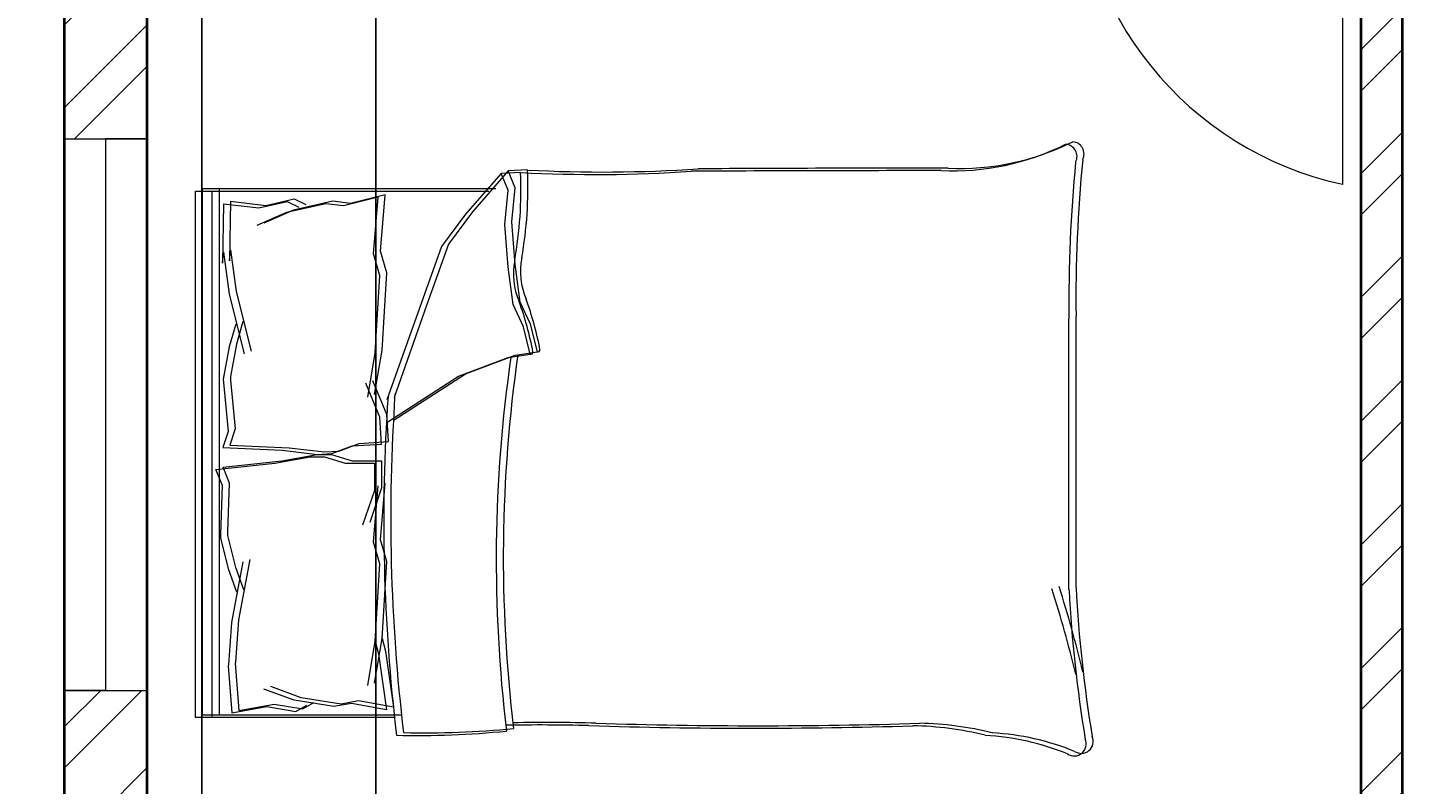
# Model space of a CAD drawing. Units: inches. Extents: x 1355 to 2746, y 1171 to 2751.
# Tile 7 of 24: x 1511 to 1663, y 1818 to 1901. Entities that reach past the tile are written whole.
import ezdxf

# ---------------------------------------------------------------- set-up
doc = ezdxf.new("R2010")
doc.units = ezdxf.units.IN
for name, color, linetype, lineweight in [('A-ANNO-DIMS', 2, 'Continuous', 18), ('A-DOOR', 3, 'Continuous', 20), ('A-FURN', 8, 'Continuous', 13), ('A-GLAZ', 4, 'Continuous', 18), ('A-WALL', 7, 'Continuous', 40), ('A-WALL-PATT', 252, 'Continuous', 13)]:
    doc.layers.add(name, color=color, linetype=linetype, lineweight=lineweight)
doc.styles.get("Standard").update_dxf_attribs({"font": 'arial.ttf'})
doc.dimstyles.get("Standard").update_dxf_attribs({"dimtxt": 0.18, "dimasz": 0.18, "dimexe": 0.18, "dimexo": 0.0625, "dimgap": 0.09, "dimtad": 0, "dimtih": 1, "dimtoh": 1, "dimdec": 4, "dimzin": 0, "dimdsep": 46, "dimtxsty": 'Standard', "dimcen": 0.09, "dimadec": 0, "dimazin": 0, "dimtfac": 1, "dimtdec": 4, "dimtofl": 0, "dimtmove": 0, "dimatfit": 3, "dimfxl": 1, "dimtolj": 1, "dimtzin": 0, "dimarcsym": 0})

# ---------------------------------------------------------------- blocks, each defined once
blk = doc.blocks.new('BED-DOUBLE-PLAN')
for p, q in [((75.16, 62.38), (96.87, 62.38)), ((75.93, 62.66), (97.64, 62.66)), ((95.03, 62.38), (95.03, 5.09)), ((95.8, 62.66), (95.8, 5.36)), ((96.87, 62.38), (96.87, 5.09)), ((97.64, 62.66), (97.64, 5.36)), ((76.95, 55.42), (76.08, 61.53)), ((76.08, 61.53), (79.9, 60.84)), ((77.72, 55.7), (76.85, 61.81)), ((76.85, 61.81), (80.66, 61.11)), ((79.9, 60.84), (81.8, 61.19)), ((80.66, 61.11), (82.57, 61.46)), ((81.8, 61.19), (86.14, 60.49)), ((82.57, 61.46), (86.9, 60.77)), ((85.96, 61.71), (84.75, 61.01)), ((86.73, 61.98), (85.52, 61.29)), ((89.08, 61.19), (85.96, 61.71)), ((89.85, 61.46), (86.73, 61.98)), ((86.9, 60.77), (90.2, 59.55)), ((92.9, 61.88), (89.08, 61.19)), ((93.66, 62.15), (89.85, 61.46)), ((92.87, 61.87), (93.27, 56.74)), ((93.64, 62.15), (94.03, 57.02)), ((86.14, 60.49), (89.43, 59.28)), ((78.14, 58.9), (77.34, 54.06)), ((78.9, 59.17), (78.1, 54.34)), ((93.24, 56.62), (92.9, 52.03)), ((93.27, 56.74), (93.24, 56.62)), ((94.01, 56.89), (93.66, 52.31)), ((94.03, 57.02), (94.01, 56.89)), ((77.34, 54.06), (76.95, 55.42)), ((78.1, 54.34), (77.72, 55.7)), ((77.34, 54.06), (76.82, 45.66)), ((78.1, 54.34), (77.59, 45.93)), ((92.9, 52.03), (91.68, 45.45)), ((93.66, 52.31), (92.45, 45.72)), ((2.64, 48.76), (2.64, 19.26)), ((92.38, 48.74), (93.24, 46.31)), ((93.14, 49.01), (94.01, 46.59)), ((1.87, 48.49), (1.87, 18.98)), ((76.82, 45.66), (77.49, 43.31)), ((77.59, 45.93), (78.25, 43.58)), ((93.24, 46.31), (94.11, 42.85)), ((94.01, 46.59), (94.88, 43.12)), ((77.49, 43.31), (77, 37.16)), ((78.25, 43.58), (77.77, 37.43)), ((94.11, 42.85), (94.11, 42.46)), ((94.88, 42.74), (94.7, 37.41)), ((94.88, 43.12), (94.88, 42.74)), ((77.38, 37.65), (78.68, 41.42)), ((78.14, 37.93), (79.45, 41.7)), ((94.11, 42.46), (93.94, 37.13)), ((77.38, 34.71), (77.38, 37.65)), ((78.14, 34.98), (78.14, 37.93)), ((93.94, 37.13), (94.63, 35.4)), ((94.7, 37.41), (95.4, 35.67)), ((81.36, 34.98), (78.14, 34.98)), ((83.61, 34.29), (81.36, 34.98)), ((88.98, 34.98), (85.17, 34.29)), ((94.63, 35.4), (88.22, 34.71)), ((95.4, 35.67), (88.98, 34.98)), ((80.59, 34.71), (77.38, 34.71)), ((82.03, 33.66), (79.83, 32.82)), ((82.84, 34.01), (80.59, 34.71)), ((82.8, 33.93), (80.6, 33.1)), ((83.59, 33.75), (82.03, 33.66)), ((84.36, 34.03), (82.8, 33.93)), ((84.4, 34.01), (82.84, 34.01)), ((87.44, 33.3), (83.59, 33.75)), ((85.17, 34.29), (83.61, 34.29)), ((88.21, 33.57), (84.36, 34.03)), ((88.22, 34.71), (84.4, 34.01)), ((94.65, 33.28), (88.21, 33.57)), ((79.83, 32.82), (76.62, 32.62)), ((76.62, 32.62), (76.8, 29.68)), ((80.6, 33.1), (77.39, 32.9)), ((77.39, 32.9), (77.57, 29.96)), ((93.89, 33.01), (87.44, 33.3)), ((93.3, 31.24), (93.89, 33.01)), ((94.07, 31.51), (94.65, 33.28)), ((76.8, 30.55), (69.01, 25.52)), ((93.81, 25.93), (93.3, 31.24)), ((94.57, 26.2), (94.07, 31.51)), ((76.03, 30.27), (68.25, 25.25)), ((76.8, 29.68), (78.34, 26)), ((77.57, 29.96), (79.11, 26.28)), ((72.52, 17.82), (76.03, 27.82)), ((73.28, 18.1), (76.8, 28.09)), ((78.14, 27.51), (77.34, 22.68)), ((78.9, 27.78), (78.1, 22.95)), ((93.83, 25.54), (93.81, 25.93)), ((93.95, 22.3), (94.6, 25.82)), ((94.6, 25.82), (94.57, 26.2)), ((68.25, 25.25), (62.87, 23.21)), ((69.01, 25.52), (63.63, 23.48)), ((93.18, 22.03), (93.83, 25.54)), ((62.87, 23.21), (60.45, 22.84)), ((60.45, 22.84), (61.2, 19.86)), ((63.63, 23.48), (61.22, 23.11)), ((61.22, 23.11), (61.96, 20.14)), ((78.1, 22.95), (77.59, 14.54)), ((93.19, 16.3), (91.57, 22.8)), ((93.96, 16.57), (92.34, 23.07)), ((77.34, 22.68), (76.82, 14.27)), ((92.47, 19.55), (93.18, 22.03)), ((93.23, 19.83), (93.95, 22.3)), ((61.2, 19.86), (62.31, 17.45)), ((61.96, 20.14), (63.08, 17.72)), ((62.31, 17.45), (62.87, 13.37)), ((63.08, 17.72), (63.63, 13.64)), ((70.1, 11.14), (72.52, 17.82)), ((70.87, 11.41), (73.28, 18.1)), ((93.82, 11.75), (93.19, 16.3)), ((94.59, 12.02), (93.96, 16.57)), ((76.82, 14.27), (77.49, 11.92)), ((77.59, 14.54), (78.25, 12.19)), ((62.87, 13.37), (63.24, 8.72)), ((63.63, 13.64), (64, 9)), ((78.25, 12.19), (77.77, 6.04)), ((93.81, 6.47), (93.92, 12.95)), ((93.92, 12.95), (93.82, 11.75)), ((94.57, 6.75), (94.69, 13.22)), ((94.69, 13.22), (94.59, 12.02)), ((67.51, 7.61), (70.1, 11.14)), ((68.27, 7.88), (70.87, 11.41)), ((77.49, 11.92), (77, 5.77)), ((87.74, 7.71), (90.95, 9.12)), ((63.24, 8.72), (62.87, 5.01)), ((63.61, 3.17), (67.51, 7.61)), ((64, 9), (63.63, 5.28)), ((64.38, 3.44), (68.27, 7.88)), ((83.46, 6.75), (87.74, 7.71)), ((86.97, 7.43), (90.18, 8.85)), ((77, 5.77), (80.77, 6.7)), ((77.77, 6.04), (81.53, 6.97)), ((80.77, 6.7), (82.69, 6.47)), ((81.53, 6.97), (83.46, 6.75)), ((82.69, 6.47), (86.97, 7.43)), ((86.88, 6.21), (85.62, 6.83)), ((87.64, 6.49), (86.39, 7.1)), ((89.96, 6.93), (86.88, 6.21)), ((90.72, 7.2), (87.64, 6.49)), ((93.81, 6.47), (89.96, 6.93)), ((94.57, 6.75), (90.72, 7.2)), ((62.87, 5.01), (63.61, 3.17)), ((63.63, 5.28), (64.38, 3.44)), ((96.87, 5.09), (64.97, 5.09)), ((97.64, 5.36), (65.74, 5.36)), ((61.52, 3.07), (63.61, 3.17, 4.64)), ((62.28, 3.35), (64.38, 3.44, 4.64))]:
    blk.add_line(p, q)
for centre, radius, start, end in [((2.07, 65.52), 1.31, 56.1736, 203.4781), ((1.3, 65.24), 1.31, 56.1736, 203.4781), ((12.62, 92.52), 28.25, 247.9751, 266.652), ((13.39, 92.79), 28.25, 247.9751, 266.652), ((-143.9, 40.86), 145.97, 2.9958, 9.4091), ((-143.14, 41.13), 145.97, 2.9958, 9.4091), ((19.53, 98.8), 35.53, 256.0648, 268.9113), ((20.29, 99.07), 35.53, 256.0648, 268.9113), ((36.96, -514.41), 578.22, 88.22771, 91.71854), ((-90.53, 45.26), 154.68, 351.7845, 6.9006), ((72.78, -35.55), 99.87, 88.7218, 95.604), ((-89.76, 45.54), 154.68, 351.7845, 6.9006), ((73.55, -35.27), 99.87, 88.7218, 95.604), ((-121.38, 40.94), 197.77, 356.0865, 6.7821), ((-120.62, 41.22), 197.77, 356.0865, 6.7821), ((36.19, -514.68), 578.22, 88.22771, 91.71854), ((59.5, 267.13), 203.94, 268.4762, 271.0082), ((60.27, 267.4), 203.94, 268.4762, 271.0082), ((126.07, 87.47), 127.63, 193.3832, 197.7053), ((125.3, 87.2), 127.63, 193.3832, 197.7053), ((60.38, 22.63), 0.221, 70.2464, 181.1377), ((61.15, 22.9), 0.221, 70.2464, 181.1377), ((95.86, 29.47), 35.55, 190.6617, 199.8806), ((95.1, 29.2), 35.55, 190.6617, 199.8806), ((-157.62, 17.21), 159.5, 354.4998, 0.6351), ((-156.85, 17.49), 159.5, 354.4998, 0.6351), ((54.83, 14.11), 7.46, 348.6608, 23.7384), ((55.6, 14.38), 7.46, 348.6608, 23.7384), ((104.85, 5.01), 43.38, 169.8763, 182.5657), ((105.62, 5.29), 43.38, 169.8763, 182.5657), ((15.32, -24.48), 27.65, 87.4714, 116.4681), ((16.33, 5472.16), 5469.02, 270.00217, 270.28689), ((53.34, -151.96), 155.25, 86.9791, 93.8365), ((54.1, -151.69), 155.25, 86.9791, 93.8365), ((2.32, 1.32), 1.32, 152.6588, 266.02), ((3.08, 1.59), 1.32, 152.6588, 266.02), ((14.55, -24.75), 27.65, 87.4714, 116.4681), ((15.56, 5471.89), 5469.02, 270.00217, 270.28689)]:
    blk.add_arc(centre, radius, start, end)
blk = doc.blocks.new('WINDOW-PLAN-60')
for p, q in [((0, 60), (9, 60)), ((9, 60), (4.5, 60)), ((4.5, 60), (4.5, 0)), ((4.5, 0), (0, 0)), ((0, 0), (9, 0))]:
    blk.add_line(p, q)
blk = doc.blocks.new('DOOR-BEDROOM-NW')
for p, q in [((0, 38.25), (0, 33.75)), ((33, 33.75), (33, 38.25)), ((0, 33.75), (0, 36)), ((0, 36), (2, 36)), ((33, 36), (31, 36)), ((31, 36), (31, 0))]:
    blk.add_line(p, q)
blk.add_arc((38.85, 36), 36.84, 180, 257.7067)
blk = doc.blocks.new('*D96')
at = {"layer": 'A-ANNO-DIMS', "color": 0, "lineweight": -2, "transparency": 16777216}
for p, q in [((1514.65, 2139.3), (1407.53, 2139.3)), ((1407.71, 2139.12), (1407.71, 1725.48)), ((1407.71, 1311.48), (1407.71, 1725.12)), ((1514.65, 1311.3), (1407.53, 1311.3))]:
    blk.add_line(p, q, dxfattribs=at)
at = {"layer": 'A-ANNO-DIMS', "color": 0, "transparency": 16777216}
for points in [[(1407.68, 2139.12), (1407.74, 2139.12), (1407.71, 2139.3)], [(1407.68, 1311.48), (1407.74, 1311.48), (1407.71, 1311.3)]]:
    blk.add_solid(points, dxfattribs=at)
at = {"layer": 'Defpoints', "color": 0, "transparency": 16777216}
for p in [(1407.71, 2139.3), (1514.71, 2139.3), (1514.71, 1311.3)]:
    blk.add_point(p, dxfattribs=at)
at = {"layer": 'A-ANNO-DIMS', "color": 0, "transparency": 16777216, "insert": (1407.71, 1725.3), "char_height": 0.18, "attachment_point": 5}
blk.add_mtext('\\A1;828', dxfattribs=at)
blk = doc.blocks.new('*D103')
at = {"layer": 'A-ANNO-DIMS', "color": 0, "lineweight": -2, "transparency": 16777216}
for p, q in [((2089.33, 1917.3), (1407.53, 1917.3)), ((1407.71, 1917.12), (1407.71, 1840.98)), ((1407.71, 1764.48), (1407.71, 1840.62)), ((2089.33, 1764.3), (1407.53, 1764.3))]:
    blk.add_line(p, q, dxfattribs=at)
at = {"layer": 'A-ANNO-DIMS', "color": 0, "transparency": 16777216}
for points in [[(1407.68, 1917.12), (1407.74, 1917.12), (1407.71, 1917.3)], [(1407.68, 1764.48), (1407.74, 1764.48), (1407.71, 1764.3)]]:
    blk.add_solid(points, dxfattribs=at)
at = {"layer": 'Defpoints', "color": 0, "transparency": 16777216}
for p in [(1407.71, 1917.3), (2089.39, 1917.3), (2089.39, 1764.3)]:
    blk.add_point(p, dxfattribs=at)
at = {"layer": 'A-ANNO-DIMS', "color": 0, "transparency": 16777216, "insert": (1407.71, 1840.8), "char_height": 0.18, "attachment_point": 5}
blk.add_mtext('\\A1;153', dxfattribs=at)
blk = doc.blocks.new('*D137')
at = {"layer": 'A-ANNO-DIMS', "color": 0, "lineweight": -2, "transparency": 16777216}
for p, q in [((1523.71, 1921.74), (1523.71, 1171.06)), ((1529.67, 1919.49), (1529.67, 1171.06)), ((1523.89, 1171.24), (1526.36, 1171.24)), ((1529.49, 1171.24), (1527.01, 1171.24))]:
    blk.add_line(p, q, dxfattribs=at)
at = {"layer": 'A-ANNO-DIMS', "color": 0, "transparency": 16777216}
for points in [[(1523.89, 1171.27), (1523.89, 1171.21), (1523.71, 1171.24)], [(1529.49, 1171.27), (1529.49, 1171.21), (1529.67, 1171.24)]]:
    blk.add_solid(points, dxfattribs=at)
at = {"layer": 'Defpoints', "color": 0, "transparency": 16777216}
for p in [(1523.71, 1921.8), (1529.67, 1919.55), (1529.67, 1171.24)]:
    blk.add_point(p, dxfattribs=at)
at = {"layer": 'A-ANNO-DIMS', "color": 0, "transparency": 16777216, "insert": (1526.69, 1171.24), "char_height": 0.18, "attachment_point": 5}
blk.add_mtext('\\A1;5.96', dxfattribs=at)
blk = doc.blocks.new('*D140')
at = {"layer": 'A-ANNO-DIMS', "color": 0, "lineweight": -2, "transparency": 16777216}
for p, q in [((1523.71, 1973.05), (1523.71, 1171.06)), ((1548.6, 1963.94), (1548.6, 1171.06)), ((1523.89, 1171.24), (1535.76, 1171.24)), ((1548.42, 1171.24), (1536.55, 1171.24))]:
    blk.add_line(p, q, dxfattribs=at)
at = {"layer": 'A-ANNO-DIMS', "color": 0, "transparency": 16777216}
for points in [[(1523.89, 1171.27), (1523.89, 1171.21), (1523.71, 1171.24)], [(1548.42, 1171.27), (1548.42, 1171.21), (1548.6, 1171.24)]]:
    blk.add_solid(points, dxfattribs=at)
at = {"layer": 'Defpoints', "color": 0, "transparency": 16777216}
for p in [(1523.71, 1973.11), (1548.6, 1964.01), (1548.6, 1171.24)]:
    blk.add_point(p, dxfattribs=at)
at = {"layer": 'A-ANNO-DIMS', "color": 0, "transparency": 16777216, "insert": (1536.15, 1171.24), "char_height": 0.18, "attachment_point": 5}
blk.add_mtext('\\A1;24.89', dxfattribs=at)

msp = doc.modelspace()

# ---------------------------------------------------------------- hatches: boundary and pattern name
at = {"layer": 'A-WALL-PATT'}
h = msp.add_hatch(dxfattribs=at)
h.set_pattern_fill('ANSI32', color=256)
h.paths.add_polyline_path([(1660.2083, 2139.3018), (1614.5977, 2139.3018), (1614.5977, 2130.3018), (1655.7083, 2130.3018), (1655.7083, 1981.8018), (1660.2083, 1981.8018), (1660.2083, 2090.7225), (1692.5832, 2090.7225), (1692.5832, 2095.2225), (1660.2083, 2095.2225)])
h.paths.add_polyline_path([(1523.7083, 2130.3018), (1554.5977, 2130.3018), (1554.5977, 2134.8018), (1554.5977, 2139.3018), (1514.7083, 2139.3018), (1514.7083, 2071.8385), (1523.7083, 2071.8385)])
h.paths.add_polyline_path([(1940.7083, 2139.3018), (1883.7928, 2139.3018), (1883.7928, 2130.3018), (1931.7083, 2130.3018), (1931.7083, 2098.3333), (1940.7083, 2098.3333)])
h.paths.add_polyline_path([(1799.7083, 2130.3018), (1823.7928, 2130.3018), (1823.7928, 2134.8018), (1823.7928, 2139.3018), (1795.2083, 2139.3018), (1795.2083, 2130.3018), (1795.2083, 2095.2225), (1759.2134, 2095.2225), (1759.2134, 2090.7225), (1795.2083, 2090.7225), (1795.2083, 1981.8018), (1799.7083, 1981.8018), (1799.7083, 1986.3018)])
h.paths.add_polyline_path([(1940.7083, 2038.3333), (1931.7083, 2038.3333), (1931.7083, 1986.3018), (1832.7083, 1986.3018), (1832.7083, 1947.1338), (1837.2083, 1947.1338), (1837.2083, 1981.8018), (1931.7083, 1981.8018), (1931.7083, 1967.1939), (1940.7083, 1967.1939)])
h.paths.add_polyline_path([(1940.7083, 1943.1939), (1931.7083, 1943.1939), (1931.7083, 1921.8018), (1837.2083, 1921.8018), (1837.2083, 1926.0511), (1832.7083, 1926.0511), (1832.7083, 1917.3018), (1931.7083, 1917.3018), (1931.7083, 1908.3321), (1940.7083, 1908.3321)])
h.paths.add_polyline_path([(1940.7083, 1884.3321), (1931.7083, 1884.3321), (1931.7083, 1869.3018), (1899.4583, 1869.3018), (1899.4583, 1864.8018), (1931.7083, 1864.8018), (1931.7083, 1773.3018), (1786.5143, 1773.3018), (1786.5143, 1764.3018), (1844.7083, 1764.3018), (1844.7083, 1748.9343), (1853.7083, 1748.9343), (1853.7083, 1764.3018), (1931.7083, 1764.3018), (1931.7083, 1652.9424), (1940.7083, 1652.9424)])
h.paths.add_polyline_path([(1799.7083, 1864.8018), (1806.0522, 1864.8018), (1806.0522, 1867.0518), (1806.0522, 1869.3018), (1799.7083, 1869.3018), (1799.7083, 1917.3018), (1799.7083, 1921.8018), (1795.2083, 1921.8018), (1795.2083, 1773.3018), (1799.7083, 1773.3018)])
h.paths.add_polyline_path([(1872.8988, 1867.0518), (1872.8988, 1869.3018), (1867.2083, 1869.3018), (1867.2083, 1917.3018), (1862.7083, 1917.3018), (1862.7083, 1869.3018), (1836.9546, 1869.3018), (1836.9546, 1864.8018), (1862.7083, 1864.8018), (1872.8988, 1864.8018)])
h.paths.add_polyline_path([(1749.2197, 1773.3018), (1655.7083, 1773.3018), (1523.7083, 1773.3018), (1523.7083, 1828.4963), (1514.7083, 1828.4963), (1514.7083, 1753.9033), (1519.2083, 1753.9033), (1523.7083, 1753.9033), (1523.7083, 1764.3018), (1655.7083, 1764.3018), (1749.2197, 1764.3018), (1749.2197, 1768.8018)])
h.paths.add_polyline_path([(1660.2083, 1921.8018), (1655.7083, 1921.8018), (1655.7083, 1917.3018), (1655.7083, 1773.3018), (1660.2083, 1773.3018)])
h.paths.add_polyline_path([(1523.7083, 2011.8385), (1514.7083, 2011.8385), (1514.7083, 1973.114), (1519.2083, 1973.114), (1523.7083, 1973.114), (1523.7083, 1976.8227), (1523.7083, 1981.8018), (1618.2083, 1981.8018), (1618.2083, 1921.8018), (1553.707, 1921.8018), (1553.707, 1917.3018), (1622.7083, 1917.3018), (1622.7083, 1919.5518), (1622.7083, 1921.8018), (1622.7083, 1986.3018), (1523.7083, 1986.3018)])
h.paths.add_polyline_path([(1529.6686, 1919.5518), (1529.6686, 1921.8018), (1523.7083, 1921.8018), (1523.7083, 1949.114), (1514.7083, 1949.114), (1514.7083, 1888.4963), (1523.7083, 1888.4963), (1523.7083, 1917.3018), (1529.6686, 1917.3018)])
h.paths.add_polyline_path([(1538.9419, 1775.643), (1585.5504, 1775.643), (1585.5504, 1798.0318), (1538.9419, 1798.0318)], flags=25)
h.paths.add_polyline_path([(1696.7097, 1497.3356), (1769.5651, 1497.3356), (1769.5651, 1523.4559), (1696.7097, 1523.4559)], flags=9)
h.paths.add_polyline_path([(1629.1643, 1230.5133), (1877.0879, 1230.5133), (1877.0879, 1267.606), (1629.1643, 1267.606)], flags=9)
h.paths.add_polyline_path([(2533.4462, 2215.4033), (2579.9292, 2215.4033), (2579.9292, 2231.889), (2533.4462, 2231.889)], flags=9)
h.paths.add_polyline_path([(2540.822, 2515.6945), (2594.2245, 2515.6945), (2594.2245, 2545.5463), (2540.822, 2545.5463)], flags=9)
h.paths.add_polyline_path([(2535.9857, 2588.2819), (2582.4687, 2588.2819), (2582.4687, 2604.7675), (2535.9857, 2604.7675)], flags=9)
h.paths.add_polyline_path([(2537.1627, 2617.1172), (2649.1245, 2617.1172), (2649.1245, 2633.6029), (2537.1627, 2633.6029)], flags=9)
h.paths.add_polyline_path([(2218.0051, 2168.228), (2363.9573, 2168.228), (2363.9573, 2205.3208), (2218.0051, 2205.3208)], flags=9)
h.paths.add_polyline_path([(1650.2156, 2165.3631), (1800.3547, 2165.3631), (1800.3547, 2202.4559), (1650.2156, 2202.4559)], flags=9)
h.paths.add_polyline_path([(2553.9592, 1610.7663), (2588.4203, 1610.7663), (2588.4203, 1660.2233), (2553.9592, 1660.2233)], flags=9)
h.paths.add_polyline_path([(1549.0868, 1648.2033), (1595.6952, 1648.2033), (1595.6952, 1670.5921), (1549.0868, 1670.5921)], flags=9)
h.paths.add_polyline_path([(1546.9525, 1502.0931), (1583.3413, 1502.0931), (1583.3413, 1524.4819), (1546.9525, 1524.4819)], flags=9)
h.paths.add_polyline_path([(1540.7704, 1433.4431), (1587.3788, 1433.4431), (1587.3788, 1455.8319), (1540.7704, 1455.8319)], flags=9)
h.paths.add_polyline_path([(1683.6524, 1321.5269), (1760.6169, 1321.5269), (1760.6169, 1333.8911), (1683.6524, 1333.8911)], flags=9)
h.paths.add_polyline_path([(1832.0485, 1356.0874), (1873.0989, 1356.0874), (1873.0989, 1378.4762), (1832.0485, 1378.4762)], flags=9)
h.paths.add_polyline_path([(1877.9694, 1431.2138), (1926.3827, 1431.2138), (1926.3827, 1453.578), (1877.9694, 1453.578)], flags=9)
h.paths.add_polyline_path([(1847.3106, 1499.8371), (1883.6994, 1499.8371), (1883.6994, 1522.2259), (1847.3106, 1522.2259)], flags=9)
h.paths.add_polyline_path([(1813.7015, 1640.7287), (1860.3099, 1640.7287), (1860.3099, 1663.1175), (1813.7015, 1663.1175)], flags=9)
h.paths.add_polyline_path([(1876.2576, 1710.2471), (1912.9452, 1710.2471), (1912.9452, 1732.6359), (1876.2576, 1732.6359)], flags=25)
h.paths.add_polyline_path([(1695.9163, 1715.3064), (1736.9668, 1715.3064), (1736.9668, 1737.6952), (1695.9163, 1737.6952)], flags=9)
h.paths.add_polyline_path([(1881.8583, 1888.9094), (1930.2717, 1888.9094), (1930.2717, 1911.2737), (1881.8583, 1911.2737)], flags=9)
h.paths.add_polyline_path([(1823.9298, 1798.6431), (1864.9803, 1798.6431), (1864.9803, 1821.0319), (1823.9298, 1821.0319)], flags=25)
h.paths.add_polyline_path([(1845.6062, 1948.1408), (1881.995, 1948.1408), (1881.995, 1970.5296), (1845.6062, 1970.5296)], flags=25)
h.paths.add_polyline_path([(1849.027, 1991.5151), (1895.6355, 1991.5151), (1895.6355, 2013.9039), (1849.027, 2013.9039)], flags=25)
h.paths.add_polyline_path([(1684.9725, 2113.8416), (1764.2658, 2113.8416), (1764.2658, 2126.2058), (1684.9725, 2126.2058)], flags=9)
h.paths.add_polyline_path([(1688.6193, 1913.0676), (1776.2005, 1913.0676), (1776.2005, 1935.4564), (1688.6193, 1935.4564)], flags=9)
h.paths.add_polyline_path([(1571.4689, 1930.9816), (1607.8577, 1930.9816), (1607.8577, 1953.3704), (1571.4689, 1953.3704)], flags=25)
h.paths.add_polyline_path([(1535.3581, 1998.3125), (1581.9665, 1998.3125), (1581.9665, 2020.7014), (1535.3581, 2020.7014)], flags=9)

# ---------------------------------------------------------------- linework, layer by layer
at = {"layer": 'A-WALL'}
for p, q in [((1514.7083, 2139.3018), (1514.7083, 1311.3018)), ((1660.2083, 1921.8018), (1660.2083, 1773.3018)), ((1523.7083, 1917.3018), (1523.7083, 1773.3018)), ((1655.7083, 1917.3018), (1655.7083, 1773.3018))]:
    msp.add_line(p, q, dxfattribs=at)

# ---------------------------------------------------------------- block references
at = {"layer": 'A-DOOR'}
msp.add_blockref('DOOR-BEDROOM-NW', (1622.708, 1883.552), dxfattribs=at)
at = {"layer": 'A-FURN', "rotation": 180}
msp.add_blockref('BED-DOUBLE-PLAN', (1626.6134, 1888.1865), dxfattribs=at)
at = {"layer": 'A-GLAZ'}
msp.add_blockref('WINDOW-PLAN-60', (1514.708, 1828.496), dxfattribs=at)

# ---------------------------------------------------------------- dimensions: what is measured, and where the dimension line sits
at = {"layer": 'A-ANNO-DIMS'}
for base, p1, p2, picture, middle in [((1407.7083, 2139.3018), (1514.7083, 1311.3018), (1514.7083, 2139.3018), '*D96', (1407.7083, 1725.3018)), ((1407.7083, 1917.3018), (2089.3909, 1764.3018), (2089.3909, 1917.3018), '*D103', (1407.7083, 1840.8018))]:
    dim = msp.add_linear_dim(base=base, p1=p1, p2=p2, angle=90, dimstyle='Standard', override={"dimdec": 0, "dimlfac": 1, "dimrnd": 0, "dimzin": 0, "dimdsep": 46, "dimlunit": 2}, dxfattribs=at)
    dim.commit()
    dim.dimension.update_dxf_attribs({"geometry": picture, "text_midpoint": middle})
for base, p1, p2, picture, middle in [((1548.5973, 1171.2388), (1523.7077, 1973.1139), (1548.5973, 1964.0069), '*D140', (1536.1525, 1171.2388)), ((1529.6686, 1171.2388), (1523.7083, 1921.8018), (1529.6686, 1919.5518), '*D137', (1526.6885, 1171.2388))]:
    dim = msp.add_linear_dim(base=base, p1=p1, p2=p2, dimstyle='Standard', override={"dimdec": 2, "dimlfac": 1, "dimrnd": 0, "dimzin": 0, "dimdsep": 46, "dimlunit": 2}, dxfattribs=at)
    dim.commit()
    dim.dimension.update_dxf_attribs({"geometry": picture, "text_midpoint": middle})

doc.saveas('drawing.dxf')
